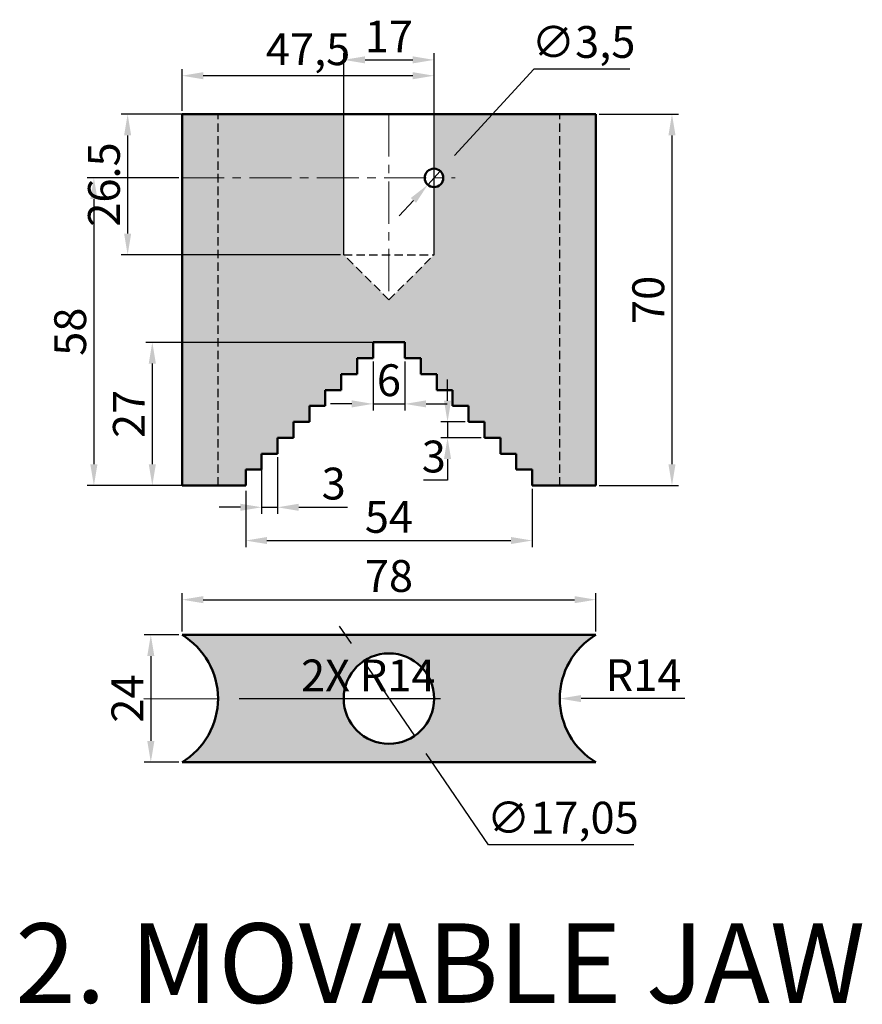
# Model space of a CAD drawing. Units: millimetres. Extents: x -14 to 1073, y -445 to 318.
# Tile 4 of 6: x 426 to 585, y 3 to 188. Entities that reach past the tile are written whole.
import ezdxf

# ---------------------------------------------------------------- set-up
doc = ezdxf.new("R2010")
doc.units = ezdxf.units.MM
doc.header["$LTSCALE"] = 0.5
doc.linetypes.add('CENTER', pattern=[50.8, 31.75, -6.35, 6.35, -6.35])
doc.linetypes.add('HIDDEN', pattern=[9.525, 6.35, -3.175])
for name, color, linetype, lineweight in [('M-CNTR', 1, 'CENTER', 18), ('M-DIMS', 2, 'Continuous', 25), ('M-HATC', 8, 'Continuous', 18), ('M-HIDN', 4, 'HIDDEN', 25), ('M-OUTL', 7, 'Continuous', 50), ('M-TEXT', 3, 'Continuous', 25)]:
    doc.layers.add(name, color=color, linetype=linetype, lineweight=lineweight)
doc.styles.get("Standard").update_dxf_attribs({"font": 'arial.ttf'})
doc.dimstyles.new('ISO-25', dxfattribs={"dimtxt": 6, "dimasz": 4, "dimexe": 1.25, "dimexo": 0.625, "dimtad": 1, "dimtoh": 1, "dimtxsty": 'Standard', "dimcen": 2.5, "dimadec": 0, "dimazin": 0, "dimtfac": 1, "dimtmove": 0, "dimatfit": 3, "dimfxl": 1, "dimarcsym": 0})

# ---------------------------------------------------------------- blocks, each defined once
blk = doc.blocks.new('*D15')
at = {"layer": 'Defpoints', "color": 0, "ltscale": 0.5, "transparency": 16777216}
for p in [(505.29, 159.68), (502.93, 157.1)]:
    blk.add_point(p, dxfattribs=at)
at = {"layer": 'M-DIMS', "color": 0, "lineweight": -2, "ltscale": 0.5, "transparency": 16777216}
for p, q in [((522.91, 178.91), (508, 162.63)), ((541.04, 178.91), (522.91, 178.91)), ((502.93, 157.1), (505.29, 159.68)), ((500.23, 154.15), (497.52, 151.21))]:
    blk.add_line(p, q, dxfattribs=at)
at = {"layer": 'M-DIMS', "color": 0, "ltscale": 0.5, "transparency": 16777216}
for points in [[(507.5, 163.08), (508.49, 162.18), (505.29, 159.68)], [(499.73, 154.6), (500.72, 153.7), (502.93, 157.1)]]:
    blk.add_solid(points, dxfattribs=at)
at = {"layer": 'M-DIMS', "color": 0, "ltscale": 0.5, "transparency": 16777216, "insert": (532.29, 183.24), "char_height": 6, "attachment_point": 5}
blk.add_mtext('∅3,5', dxfattribs=at)
blk = doc.blocks.new('*D16')
at = {"layer": 'Defpoints', "color": 0, "ltscale": 0.5, "transparency": 16777216}
for p in [(456.61, 177.65), (456.61, 170.39), (504.11, 170.39)]:
    blk.add_point(p, dxfattribs=at)
at = {"layer": 'M-DIMS', "color": 0, "lineweight": -2, "ltscale": 0.5, "transparency": 16777216}
for p, q in [((456.61, 171.02), (456.61, 178.9)), ((504.11, 171.02), (504.11, 178.9)), ((500.11, 177.65), (460.61, 177.65))]:
    blk.add_line(p, q, dxfattribs=at)
at = {"layer": 'M-DIMS', "color": 0, "ltscale": 0.5, "transparency": 16777216}
for points in [[(460.61, 178.32), (460.61, 176.99), (456.61, 177.65)], [(500.11, 178.32), (500.11, 176.99), (504.11, 177.65)]]:
    blk.add_solid(points, dxfattribs=at)
at = {"layer": 'M-DIMS', "color": 0, "ltscale": 0.5, "transparency": 16777216, "insert": (480.36, 181.87), "char_height": 6, "attachment_point": 5}
blk.add_mtext('47,5', dxfattribs=at)
blk = doc.blocks.new('*D17')
at = {"layer": 'Defpoints', "color": 0, "ltscale": 0.5, "transparency": 16777216}
for p in [(534.61, 170.39), (534.61, 100.39), (548.96, 100.39)]:
    blk.add_point(p, dxfattribs=at)
at = {"layer": 'M-DIMS', "color": 0, "lineweight": -2, "ltscale": 0.5, "transparency": 16777216}
for p, q in [((535.24, 170.39), (550.21, 170.39)), ((548.96, 166.39), (548.96, 104.39)), ((535.24, 100.39), (550.21, 100.39))]:
    blk.add_line(p, q, dxfattribs=at)
at = {"layer": 'M-DIMS', "color": 0, "ltscale": 0.5, "transparency": 16777216}
for points in [[(548.29, 166.39), (549.63, 166.39), (548.96, 170.39)], [(548.29, 104.39), (549.63, 104.39), (548.96, 100.39)]]:
    blk.add_solid(points, dxfattribs=at)
at = {"layer": 'M-DIMS', "color": 0, "ltscale": 0.5, "transparency": 16777216, "insert": (545.27, 135.39), "char_height": 6, "attachment_point": 5, "rotation": 90}
blk.add_mtext('70', dxfattribs=at)
blk = doc.blocks.new('*D18')
at = {"layer": 'Defpoints', "color": 0, "ltscale": 0.5, "transparency": 16777216}
for p in [(492.61, 124.39), (498.61, 124.39), (498.61, 115.78)]:
    blk.add_point(p, dxfattribs=at)
at = {"layer": 'M-DIMS', "color": 0, "lineweight": -2, "ltscale": 0.5, "transparency": 16777216}
for p, q in [((492.61, 123.77), (492.61, 114.53)), ((498.61, 123.77), (498.61, 114.53)), ((488.61, 115.78), (484.61, 115.78)), ((492.61, 115.78), (498.61, 115.78)), ((502.61, 115.78), (506.61, 115.78))]:
    blk.add_line(p, q, dxfattribs=at)
at = {"layer": 'M-DIMS', "color": 0, "ltscale": 0.5, "transparency": 16777216}
for points in [[(488.61, 116.45), (488.61, 115.12), (492.61, 115.78)], [(502.61, 116.45), (502.61, 115.12), (498.61, 115.78)]]:
    blk.add_solid(points, dxfattribs=at)
at = {"layer": 'M-DIMS', "color": 0, "ltscale": 0.5, "transparency": 16777216, "insert": (495.61, 119.47), "char_height": 6, "attachment_point": 5}
blk.add_mtext('6', dxfattribs=at)
blk = doc.blocks.new('*D19')
at = {"layer": 'Defpoints', "color": 0, "ltscale": 0.5, "transparency": 16777216}
for p in [(471.61, 106.39), (474.61, 106.39), (474.61, 96.29)]:
    blk.add_point(p, dxfattribs=at)
at = {"layer": 'M-DIMS', "color": 0, "lineweight": -2, "ltscale": 0.5, "transparency": 16777216}
for p, q in [((471.61, 105.77), (471.61, 95.04)), ((474.61, 105.77), (474.61, 95.04)), ((467.61, 96.29), (463.61, 96.29)), ((471.61, 96.29), (474.61, 96.29)), ((478.61, 96.29), (487.79, 96.29))]:
    blk.add_line(p, q, dxfattribs=at)
at = {"layer": 'M-DIMS', "color": 0, "ltscale": 0.5, "transparency": 16777216}
for points in [[(467.61, 96.96), (467.61, 95.62), (471.61, 96.29)], [(478.61, 96.96), (478.61, 95.62), (474.61, 96.29)]]:
    blk.add_solid(points, dxfattribs=at)
at = {"layer": 'M-DIMS', "color": 0, "ltscale": 0.5, "transparency": 16777216, "insert": (485.2, 99.98), "char_height": 6, "attachment_point": 5}
blk.add_mtext('3', dxfattribs=at)
blk = doc.blocks.new('*D20')
at = {"layer": 'Defpoints', "color": 0, "ltscale": 0.5, "transparency": 16777216}
for p in [(510.61, 112.39), (506.66, 109.39), (513.61, 109.39)]:
    blk.add_point(p, dxfattribs=at)
at = {"layer": 'M-DIMS', "color": 0, "lineweight": -2, "ltscale": 0.5, "transparency": 16777216}
for p, q in [((506.66, 116.39), (506.66, 120.39)), ((509.99, 112.39), (505.41, 112.39)), ((506.66, 112.39), (506.66, 109.39)), ((512.99, 109.39), (505.41, 109.39)), ((506.66, 105.39), (506.66, 101.39)), ((506.66, 101.39), (502.1, 101.39))]:
    blk.add_line(p, q, dxfattribs=at)
at = {"layer": 'M-DIMS', "color": 0, "ltscale": 0.5, "transparency": 16777216}
for points in [[(505.99, 116.39), (507.33, 116.39), (506.66, 112.39)], [(505.99, 105.39), (507.33, 105.39), (506.66, 109.39)]]:
    blk.add_solid(points, dxfattribs=at)
at = {"layer": 'M-DIMS', "color": 0, "ltscale": 0.5, "transparency": 16777216, "insert": (504.07, 105.08), "char_height": 6, "attachment_point": 5}
blk.add_mtext('3', dxfattribs=at)
blk = doc.blocks.new('*D21')
at = {"layer": 'Defpoints', "color": 0, "ltscale": 0.5, "transparency": 16777216}
for p in [(522.61, 100.39), (468.61, 100.04), (522.61, 90.02)]:
    blk.add_point(p, dxfattribs=at)
at = {"layer": 'M-DIMS', "color": 0, "lineweight": -2, "ltscale": 0.5, "transparency": 16777216}
for p, q in [((468.61, 99.41), (468.61, 88.77)), ((522.61, 99.77), (522.61, 88.77)), ((472.61, 90.02), (518.61, 90.02))]:
    blk.add_line(p, q, dxfattribs=at)
at = {"layer": 'M-DIMS', "color": 0, "ltscale": 0.5, "transparency": 16777216}
for points in [[(472.61, 90.69), (472.61, 89.36), (468.61, 90.02)], [(518.61, 90.69), (518.61, 89.36), (522.61, 90.02)]]:
    blk.add_solid(points, dxfattribs=at)
at = {"layer": 'M-DIMS', "color": 0, "ltscale": 0.5, "transparency": 16777216, "insert": (495.61, 93.7), "char_height": 6, "attachment_point": 5}
blk.add_mtext('54', dxfattribs=at)
blk = doc.blocks.new('*D22')
at = {"layer": 'Defpoints', "color": 0, "ltscale": 0.5, "transparency": 16777216}
for p in [(456.61, 158.39), (440, 100.39), (456.61, 100.39)]:
    blk.add_point(p, dxfattribs=at)
at = {"layer": 'M-DIMS', "color": 0, "lineweight": -2, "ltscale": 0.5, "transparency": 16777216}
for p, q in [((455.99, 158.39), (438.75, 158.39)), ((440, 154.39), (440, 104.39)), ((455.99, 100.39), (438.75, 100.39))]:
    blk.add_line(p, q, dxfattribs=at)
at = {"layer": 'M-DIMS', "color": 0, "ltscale": 0.5, "transparency": 16777216}
for points in [[(439.33, 154.39), (440.67, 154.39), (440, 158.39)], [(439.33, 104.39), (440.67, 104.39), (440, 100.39)]]:
    blk.add_solid(points, dxfattribs=at)
at = {"layer": 'M-DIMS', "color": 0, "ltscale": 0.5, "transparency": 16777216, "insert": (436.31, 129.39), "char_height": 6, "attachment_point": 5, "rotation": 90}
blk.add_mtext('58', dxfattribs=at)
blk = doc.blocks.new('*D23')
at = {"layer": 'Defpoints', "color": 0, "ltscale": 0.5, "transparency": 16777216}
for p in [(495.61, 127.39), (451.01, 100.39), (468.61, 100.39)]:
    blk.add_point(p, dxfattribs=at)
at = {"layer": 'M-DIMS', "color": 0, "lineweight": -2, "ltscale": 0.5, "transparency": 16777216}
for p, q in [((494.99, 127.39), (449.76, 127.39)), ((451.01, 123.39), (451.01, 104.39)), ((467.99, 100.39), (449.76, 100.39))]:
    blk.add_line(p, q, dxfattribs=at)
at = {"layer": 'M-DIMS', "color": 0, "ltscale": 0.5, "transparency": 16777216}
for points in [[(450.34, 123.39), (451.68, 123.39), (451.01, 127.39)], [(450.34, 104.39), (451.68, 104.39), (451.01, 100.39)]]:
    blk.add_solid(points, dxfattribs=at)
at = {"layer": 'M-DIMS', "color": 0, "ltscale": 0.5, "transparency": 16777216, "insert": (447.37, 113.89), "char_height": 6, "attachment_point": 5, "rotation": 90}
blk.add_mtext('27', dxfattribs=at)
blk = doc.blocks.new('*D24')
at = {"layer": 'Defpoints', "color": 0, "ltscale": 0.5, "transparency": 16777216}
for p in [(456.61, 72.23), (450.73, 48.23), (456.61, 48.23)]:
    blk.add_point(p, dxfattribs=at)
at = {"layer": 'M-DIMS', "color": 0, "lineweight": -2, "ltscale": 0.5, "transparency": 16777216}
for p, q in [((455.99, 72.23), (449.48, 72.23)), ((450.73, 68.23), (450.73, 52.23)), ((455.99, 48.23), (449.48, 48.23))]:
    blk.add_line(p, q, dxfattribs=at)
at = {"layer": 'M-DIMS', "color": 0, "ltscale": 0.5, "transparency": 16777216}
for points in [[(450.06, 68.23), (451.4, 68.23), (450.73, 72.23)], [(450.06, 52.23), (451.4, 52.23), (450.73, 48.23)]]:
    blk.add_solid(points, dxfattribs=at)
at = {"layer": 'M-DIMS', "color": 0, "ltscale": 0.5, "transparency": 16777216, "insert": (447.09, 60.23), "char_height": 6, "attachment_point": 5, "rotation": 90}
blk.add_mtext('24', dxfattribs=at)
blk = doc.blocks.new('*D25')
at = {"layer": 'Defpoints', "color": 0, "ltscale": 0.5, "transparency": 16777216}
for p in [(534.61, 78.87), (456.61, 72.23), (534.61, 72.23)]:
    blk.add_point(p, dxfattribs=at)
at = {"layer": 'M-DIMS', "color": 0, "lineweight": -2, "ltscale": 0.5, "transparency": 16777216}
for p, q in [((456.61, 72.85), (456.61, 80.12)), ((534.61, 72.85), (534.61, 80.12)), ((460.61, 78.87), (530.61, 78.87))]:
    blk.add_line(p, q, dxfattribs=at)
at = {"layer": 'M-DIMS', "color": 0, "ltscale": 0.5, "transparency": 16777216}
for points in [[(460.61, 79.54), (460.61, 78.21), (456.61, 78.87)], [(530.61, 79.54), (530.61, 78.21), (534.61, 78.87)]]:
    blk.add_solid(points, dxfattribs=at)
at = {"layer": 'M-DIMS', "color": 0, "ltscale": 0.5, "transparency": 16777216, "insert": (495.61, 82.56), "char_height": 6, "attachment_point": 5}
blk.add_mtext('78', dxfattribs=at)
blk = doc.blocks.new('*D26')
at = {"layer": 'Defpoints', "color": 0, "ltscale": 0.5, "transparency": 16777216}
for p in [(490.82, 67.27), (500.41, 53.18)]:
    blk.add_point(p, dxfattribs=at)
at = {"layer": 'M-DIMS', "color": 0, "lineweight": -2, "ltscale": 0.5, "transparency": 16777216}
for p, q in [((488.57, 70.58), (486.32, 73.89)), ((490.82, 67.27), (500.41, 53.18)), ((514.35, 32.68), (502.65, 49.87)), ((541.79, 32.68), (514.35, 32.68))]:
    blk.add_line(p, q, dxfattribs=at)
at = {"layer": 'M-DIMS', "color": 0, "ltscale": 0.5, "transparency": 16777216}
for points in [[(489.12, 70.96), (488.02, 70.21), (490.82, 67.27)], [(503.21, 50.24), (502.1, 49.49), (500.41, 53.18)]]:
    blk.add_solid(points, dxfattribs=at)
at = {"layer": 'M-DIMS', "color": 0, "ltscale": 0.5, "transparency": 16777216, "insert": (528.38, 37), "char_height": 6, "attachment_point": 5}
blk.add_mtext('∅17,05', dxfattribs=at)
blk = doc.blocks.new('*D27')
at = {"layer": 'Defpoints', "color": 0, "ltscale": 0.5, "transparency": 16777216}
for p in [(527.82, 60.23), (541.82, 60.23)]:
    blk.add_point(p, dxfattribs=at)
at = {"layer": 'M-DIMS', "color": 0, "lineweight": -2, "ltscale": 0.5, "transparency": 16777216}
blk.add_line((551.38, 60.23), (531.82, 60.23), dxfattribs=at)
at = {"layer": 'M-DIMS', "color": 0, "ltscale": 0.5, "transparency": 16777216}
blk.add_solid([(531.82, 60.89), (531.82, 59.56), (527.82, 60.23)], dxfattribs=at)
at = {"layer": 'M-DIMS', "color": 0, "ltscale": 0.5, "transparency": 16777216, "insert": (543.6, 63.86), "char_height": 6, "attachment_point": 5}
blk.add_mtext('R14', dxfattribs=at)
blk = doc.blocks.new('*D77')
at = {"layer": 'Defpoints', "color": 0, "ltscale": 0.5, "transparency": 16777216}
for p in [(504.11, 180.64), (487.11, 143.89), (504.11, 143.89)]:
    blk.add_point(p, dxfattribs=at)
at = {"layer": 'M-DIMS', "color": 0, "lineweight": -2, "ltscale": 0.5, "transparency": 16777216}
for p, q in [((487.11, 144.52), (487.11, 181.89)), ((491.11, 180.64), (500.11, 180.64)), ((504.11, 144.52), (504.11, 181.89))]:
    blk.add_line(p, q, dxfattribs=at)
at = {"layer": 'M-DIMS', "color": 0, "ltscale": 0.5, "transparency": 16777216}
for points in [[(491.11, 181.31), (491.11, 179.98), (487.11, 180.64)], [(500.11, 181.31), (500.11, 179.98), (504.11, 180.64)]]:
    blk.add_solid(points, dxfattribs=at)
at = {"layer": 'M-DIMS', "color": 0, "ltscale": 0.5, "transparency": 16777216, "insert": (495.61, 184.28), "char_height": 6, "attachment_point": 5}
blk.add_mtext('17', dxfattribs=at)
blk = doc.blocks.new('*D78')
at = {"layer": 'Defpoints', "color": 0, "ltscale": 0.5, "transparency": 16777216}
for p in [(487.11, 170.39), (446.36, 143.89), (487.11, 143.89)]:
    blk.add_point(p, dxfattribs=at)
at = {"layer": 'M-DIMS', "color": 0, "lineweight": -2, "ltscale": 0.5, "transparency": 16777216}
for p, q in [((486.49, 170.39), (445.11, 170.39)), ((446.36, 166.39), (446.36, 147.89)), ((486.49, 143.89), (445.11, 143.89))]:
    blk.add_line(p, q, dxfattribs=at)
at = {"layer": 'M-DIMS', "color": 0, "ltscale": 0.5, "transparency": 16777216}
for points in [[(445.69, 166.39), (447.03, 166.39), (446.36, 170.39)], [(445.69, 147.89), (447.03, 147.89), (446.36, 143.89)]]:
    blk.add_solid(points, dxfattribs=at)
at = {"layer": 'M-DIMS', "color": 0, "ltscale": 0.5, "transparency": 16777216, "insert": (442.67, 157.14), "char_height": 6, "attachment_point": 5, "rotation": 90}
blk.add_mtext('26.5', dxfattribs=at)
blk = doc.blocks.new('*D84')
at = {"layer": 'Defpoints', "color": 0, "ltscale": 0.5, "transparency": 16777216}
for p in [(449.4, 60.23), (463.4, 60.2)]:
    blk.add_point(p, dxfattribs=at)
at = {"layer": 'M-DIMS', "color": 0, "lineweight": -2, "ltscale": 0.5, "transparency": 16777216}
for p, q in [((449.4, 60.23), (463.4, 60.2)), ((477.43, 60.17), (467.4, 60.19)), ((505.36, 60.17), (477.43, 60.17))]:
    blk.add_line(p, q, dxfattribs=at)
at = {"layer": 'M-DIMS', "color": 0, "ltscale": 0.5, "transparency": 16777216}
blk.add_solid([(467.4, 60.86), (467.4, 59.53), (463.4, 60.2)], dxfattribs=at)
at = {"layer": 'M-DIMS', "color": 0, "ltscale": 0.5, "transparency": 16777216, "insert": (491.71, 63.81), "char_height": 6, "attachment_point": 5}
blk.add_mtext('2X R14', dxfattribs=at)

msp = doc.modelspace()

# ---------------------------------------------------------------- hatches: boundary and pattern name
at = {"layer": 'M-HATC', "ltscale": 0.5}
h = msp.add_hatch(color=256, dxfattribs=at)
h.set_gradient(color1=(41, 49, 137), color2=(41, 49, 137), tint=1)
h.paths.add_polyline_path([(487.1109, 158.3935), (463.3998, 158.3935), (463.3998, 100.3935), (468.6109, 100.3935), (468.6109, 103.3935), (471.6109, 103.3935), (471.6109, 106.3935), (474.6109, 106.3935), (474.6109, 109.3935), (477.6109, 109.3935), (477.6109, 112.3935), (480.6109, 112.3935), (480.6109, 115.3935), (483.6109, 115.3935), (483.6109, 118.3935), (486.6109, 118.3935), (486.6109, 121.3935), (489.6109, 121.3935), (489.6109, 124.3935), (492.6109, 124.3935), (492.6109, 127.3935), (498.6109, 127.3935), (498.6109, 124.3935), (501.6109, 124.3935), (501.6109, 121.3935), (504.6109, 121.3935), (504.6109, 118.3935), (507.6109, 118.3935), (507.6109, 115.3935), (510.6109, 115.3935), (510.6109, 112.3935), (513.6109, 112.3935), (513.6109, 109.3935), (516.6109, 109.3935), (516.6109, 106.3935), (519.6109, 106.3935), (519.6109, 103.3935), (522.6109, 103.3935), (522.6109, 100.3935), (527.822, 100.3935), (527.822, 170.3935), (504.1109, 170.3935), (504.1109, 160.1435, -0.41421356), (505.8609, 158.3935, -0.41421356), (504.1109, 156.6435), (504.1109, 143.8935), (495.6109, 135.3935), (487.1109, 143.8935)])
h.paths.add_polyline_path([(487.1109, 170.3935), (463.3998, 170.3935), (463.3998, 158.3935), (487.1109, 158.3935)], flags=17)
h.paths.add_polyline_path([(534.6109, 170.3935), (527.822, 170.3935), (527.822, 100.3935), (534.6109, 100.3935)])
h.paths.add_polyline_path([(463.3998, 158.3935), (456.6109, 158.3935), (456.6109, 100.3935), (463.3998, 100.3935)])
h.paths.add_polyline_path([(463.3998, 170.3935), (456.6109, 170.3935), (456.6109, 158.3935), (463.3998, 158.3935)])
h = msp.add_hatch(color=256, dxfattribs=at)
h.set_gradient(color1=(69, 84, 165), color2=(41, 49, 137), tint=1)
h.paths.add_polyline_path([(534.6109, 48.2255, -0.56574145), (534.6109, 72.2255), (456.6109, 72.2255, -0.56574145), (456.6109, 48.2255)])
h.paths.add_polyline_path([(487.0859, 60.2255, -1), (504.1359, 60.2255, -1)], flags=16)

# ---------------------------------------------------------------- linework, layer by layer
at = {"layer": 'M-CNTR', "ltscale": 0.5}
for p, q in [((495.6109, 170.3935), (495.6109, 135.3935)), ((456.6109, 158.3935), (508.1114, 158.3935))]:
    msp.add_line(p, q, dxfattribs=at)
at = {"layer": 'M-HIDN', "ltscale": 0.5}
for p, q in [((463.3998, 100.3935), (463.3998, 170.3935)), ((487.1109, 143.8935), (487.1109, 170.3935)), ((504.1109, 143.8935), (504.1109, 170.3935)), ((527.822, 100.3935), (527.822, 170.3935)), ((495.6109, 135.3935), (487.1109, 143.8935)), ((487.1109, 143.8935), (504.1109, 143.8935)), ((495.6109, 135.3935), (504.1109, 143.8935))]:
    msp.add_line(p, q, dxfattribs=at)
at = {"layer": 'M-OUTL', "ltscale": 0.5}
for p, q in [((456.6109, 170.3935), (534.6109, 170.3935)), ((456.6109, 100.3935), (456.6109, 170.3935)), ((534.6109, 170.3935), (534.6109, 100.3935)), ((498.6109, 127.3935), (492.6109, 127.3935)), ((492.6109, 127.3935), (492.6109, 124.3935)), ((498.6109, 127.3935), (498.6109, 124.3935)), ((492.6109, 124.3935), (489.6109, 124.3935)), ((489.6109, 124.3935), (489.6109, 121.3935)), ((498.6109, 124.3935), (501.6109, 124.3935)), ((501.6109, 124.3935), (501.6109, 121.3935)), ((489.6109, 121.3935), (486.6109, 121.3935)), ((486.6109, 121.3935), (486.6109, 118.3935)), ((501.6109, 121.3935), (504.6109, 121.3935)), ((504.6109, 121.3935), (504.6109, 118.3935)), ((486.6109, 118.3935), (483.6109, 118.3935)), ((483.6109, 118.3935), (483.6109, 115.3935)), ((504.6109, 118.3935), (507.6109, 118.3935)), ((507.6109, 118.3935), (507.6109, 115.3935)), ((483.6109, 115.3935), (480.6109, 115.3935)), ((480.6109, 115.3935), (480.6109, 112.3935)), ((507.6109, 115.3935), (510.6109, 115.3935)), ((510.6109, 115.3935), (510.6109, 112.3935)), ((480.6109, 112.3935), (477.6109, 112.3935)), ((477.6109, 112.3935), (477.6109, 109.3935)), ((510.6109, 112.3935), (513.6109, 112.3935)), ((513.6109, 112.3935), (513.6109, 109.3935)), ((477.6109, 109.3935), (474.6109, 109.3935)), ((474.6109, 109.3935), (474.6109, 106.3935)), ((513.6109, 109.3935), (516.6109, 109.3935)), ((516.6109, 109.3935), (516.6109, 106.3935)), ((474.6109, 106.3935), (471.6109, 106.3935)), ((471.6109, 106.3935), (471.6109, 103.3935)), ((516.6109, 106.3935), (519.6109, 106.3935)), ((519.6109, 106.3935), (519.6109, 103.3935)), ((468.6109, 103.3935), (468.6109, 100.3935)), ((471.6109, 103.3935), (468.6109, 103.3935)), ((519.6109, 103.3935), (522.6109, 103.3935)), ((522.6109, 103.3935), (522.6109, 100.3935)), ((468.6109, 100.3935), (456.6109, 100.3935)), ((534.6109, 100.3935), (522.6109, 100.3935)), ((456.6109, 72.2255), (534.6109, 72.2255)), ((534.6109, 48.2255), (456.6109, 48.2255))]:
    msp.add_line(p, q, dxfattribs=at)
for centre, radius in [((504.1109, 158.3935), 1.75), ((495.6109, 60.2255), 8.525)]:
    msp.add_circle(centre, radius, dxfattribs=at)
for centre, start, end in [((449.3998, 60.2255), 301.002719, 58.997281), ((541.822, 60.2255), 121.002719, 238.997281)]:
    msp.add_arc(centre, 14, start, end, dxfattribs=at)

# ---------------------------------------------------------------- texts
at = {"layer": 'M-TEXT', "ltscale": 0.5, "insert": (418.2374, 17.854), "char_height": 15, "attachment_point": 1}
msp.add_mtext_dynamic_manual_height_columns('\\pxqc;2. MOVABLE JAW', width=174.108625, gutter_width=12.5, heights=[0], dxfattribs=at)

# ---------------------------------------------------------------- dimensions: what is measured, and where the dimension line sits
at = {"layer": 'M-DIMS', "ltscale": 0.5}
for base, p1, p2, override, picture, middle in [((504.1109, 180.6435), (487.1109, 143.8935), (504.1109, 143.8935), {"dimdec": 0, "dimlfac": 1, "dimrnd": 0, "dimzin": 0, "dimdsep": 46, "dimlunit": 2}, '*D77', (495.6109, 184.2808)), ((456.6109, 177.6538), (504.1109, 170.3935), (456.6109, 170.3935), {"dimclrd": 0, "dimclre": 0, "dimclrt": 0}, '*D16', (480.3609, 181.8723)), ((498.6109, 115.784), (492.6109, 124.3935), (498.6109, 124.3935), {"dimclrd": 0, "dimclre": 0, "dimclrt": 0}, '*D18', (495.6109, 119.4725)), ((474.6109, 96.2891), (471.6109, 106.3935), (474.6109, 106.3935), {"dimclrd": 0, "dimclre": 0, "dimclrt": 0}, '*D19', (485.2005, 99.9796)), ((522.6109, 90.0243), (468.6109, 100.0391), (522.6109, 100.3935), {"dimclrd": 0, "dimclre": 0, "dimclrt": 0}, '*D21', (495.6109, 93.7005)), ((534.6109, 78.8724), (456.6109, 72.2255), (534.6109, 72.2255), {"dimclrd": 0, "dimclre": 0, "dimclrt": 0}, '*D25', (495.6109, 82.5609))]:
    dim = msp.add_linear_dim(base=base, p1=p1, p2=p2, dimstyle='ISO-25', override=override, dxfattribs=at)
    dim.commit()
    dim.dimension.update_dxf_attribs({"geometry": picture, "text_midpoint": middle})
for p1, p2, picture, middle in [((502.9286, 157.1034), (505.2933, 159.6837), '*D15', (532.2869, 178.9104)), ((490.8165, 67.2746), (500.4054, 53.1765), '*D26', (528.3839, 32.6757))]:
    dim = msp.add_diameter_dim_2p(p1=p1, p2=p2, dimstyle='ISO-25', override={"dimclrd": 0, "dimclre": 0, "dimclrt": 0}, dxfattribs=at)
    dim.commit()
    dim.dimension.update_dxf_attribs({"geometry": picture, "text_midpoint": middle, "dimtype": 163})
for base, p1, p2, override, picture, middle in [((446.3609, 143.8935), (487.1109, 170.3935), (487.1109, 143.8935), {"dimdec": 1, "dimlfac": 1, "dimrnd": 0, "dimzin": 0, "dimdsep": 46, "dimlunit": 2}, '*D78', (442.6725, 157.1435)), ((548.9588, 100.3935), (534.6109, 170.3935), (534.6109, 100.3935), {"dimclrd": 0, "dimclre": 0, "dimclrt": 0}, '*D17', (545.2704, 135.3935)), ((439.999, 100.3935), (456.6109, 158.3935), (456.6109, 100.3935), {"dimclrd": 0, "dimclre": 0, "dimclrt": 0}, '*D22', (436.3106, 129.3935)), ((451.0091, 100.3935), (495.6109, 127.3935), (468.6109, 100.3935), {"dimclrd": 0, "dimclre": 0, "dimclrt": 0}, '*D23', (447.3718, 113.8935)), ((506.6587, 109.3935), (510.6109, 112.3935), (513.6109, 109.3935), {"dimclrd": 0, "dimclre": 0, "dimclrt": 0}, '*D20', (504.0692, 105.084)), ((450.7296, 48.2255), (456.6109, 72.2255), (456.6109, 48.2255), {"dimclrd": 0, "dimclre": 0, "dimclrt": 0}, '*D24', (447.0923, 60.2255))]:
    dim = msp.add_linear_dim(base=base, p1=p1, p2=p2, angle=90, dimstyle='ISO-25', override=override, dxfattribs=at)
    dim.commit()
    dim.dimension.update_dxf_attribs({"geometry": picture, "text_midpoint": middle})
dim = msp.add_radius_dim(center=(449.3998, 60.2255), mpoint=(463.3998, 60.2), text='2X <>', dimstyle='ISO-25', override={"dimdec": 0, "dimlfac": 1, "dimrnd": 0, "dimzin": 0, "dimdsep": 46, "dimlunit": 2}, dxfattribs=at)
dim.commit()
dim.dimension.update_dxf_attribs({"geometry": '*D84', "text_midpoint": (491.7069, 63.8138)})
dim = msp.add_radius_dim(center=(541.822, 60.2255), mpoint=(527.822, 60.2255), dimstyle='ISO-25', override={"dimclrd": 0, "dimclre": 0, "dimclrt": 0}, dxfattribs=at)
dim.commit()
dim.dimension.update_dxf_attribs({"geometry": '*D27', "text_midpoint": (543.6032, 60.2255), "dimtype": 164})

doc.saveas('drawing.dxf')
